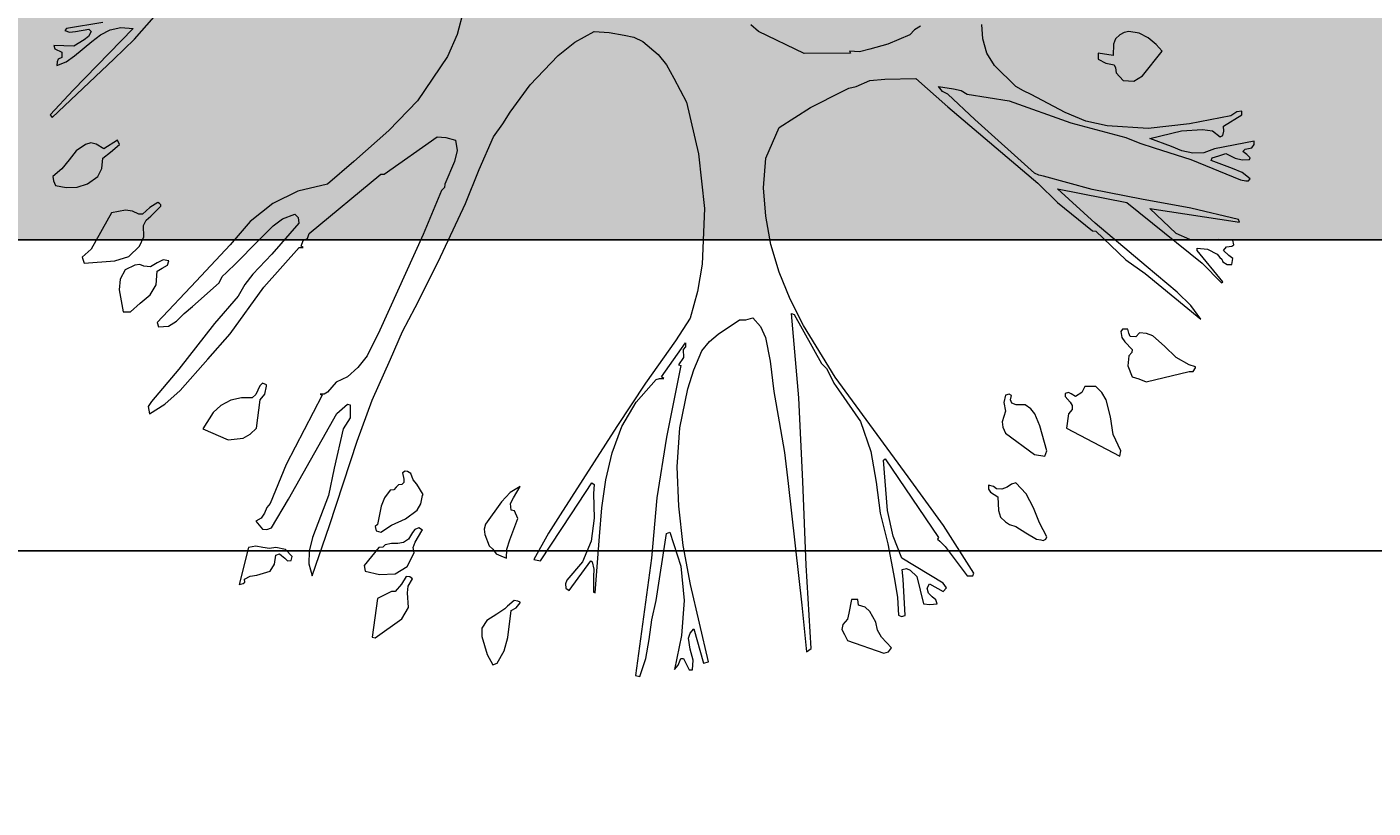
# Model space of a CAD drawing. Units: inches. Extents: x 84 to 1044, y -280 to 906.
# Tile 37 of 105: x 876 to 915, y -129 to -107. Entities that reach past the tile are written whole.
import ezdxf

# ---------------------------------------------------------------- set-up
doc = ezdxf.new("R2010")
doc.units = ezdxf.units.IN
for name, color, linetype, lineweight in [('A-ANNO-DIMS', 2, 'Continuous', 18), ('C-PROP', 7, 'Continuous', 25), ('L-PLNT', 114, 'Continuous', 15)]:
    doc.layers.add(name, color=color, linetype=linetype, lineweight=lineweight)
doc.layers.add('L-PLNT-PATT', color=9, linetype='Continuous', lineweight=9, true_color=0xafd9aa)
doc.styles.get("Standard").update_dxf_attribs({"font": 'arial.ttf'})
doc.dimstyles.get("Standard").update_dxf_attribs({"dimtxt": 0.18, "dimasz": 0.18, "dimexe": 0.18, "dimexo": 0.0625, "dimgap": 0.09, "dimtad": 0, "dimtih": 1, "dimtoh": 1, "dimdec": 4, "dimzin": 0, "dimdsep": 46, "dimtxsty": 'Standard', "dimcen": 0.09, "dimadec": 0, "dimazin": 0, "dimtfac": 1, "dimtdec": 4, "dimtofl": 0, "dimtmove": 0, "dimatfit": 3, "dimfxl": 1, "dimtolj": 1, "dimtzin": 0, "dimarcsym": 0})

# ---------------------------------------------------------------- blocks, each defined once
blk = doc.blocks.new('A$C37E508DF')
for p, q in [((0.9287, 0.7825), (0.936, 0.7542)), ((1.3151, 0.7487), (1.2919, 0.7752)), ((0.3186, 0.7491), (0.3199, 0.7662)), ((0.3919, 0.7641), (0.3988, 0.7598)), ((0.3988, 0.7598), (0.4043, 0.7538)), ((0.5823, 0.7577), (0.5913, 0.7658)), ((1.3309, 0.7624), (1.3164, 0.7615)), ((1.3164, 0.7615), (1.3871, 0.6891)), ((1.3434, 0.7598), (1.3309, 0.7624)), ((1.355, 0.7538), (1.3434, 0.7598)), ((1.352, 0.7684), (1.3948, 0.7615)), ((1.3687, 0.7607), (1.3657, 0.7577)), ((1.3841, 0.7577), (1.3687, 0.7607)), ((1.397, 0.759), (1.3914, 0.7572)), ((1.3948, 0.7615), (1.397, 0.759)), ((0.1153, 0.7427), (0.1244, 0.7504)), ((0.1244, 0.7504), (0.1351, 0.7559)), ((0.1351, 0.7559), (0.1471, 0.7577)), ((0.1471, 0.7577), (0.1527, 0.7568)), ((0.1527, 0.7568), (0.1578, 0.7538)), ((0.1578, 0.7538), (0.1629, 0.7491)), ((0.1629, 0.7491), (0.1651, 0.7431)), ((0.1651, 0.7431), (0.1655, 0.7298)), ((0.3139, 0.7324), (0.3186, 0.7491)), ((0.4043, 0.7538), (0.4301, 0.7431)), ((0.4301, 0.7431), (0.4515, 0.7371)), ((0.5287, 0.7319), (0.5823, 0.7577)), ((0.7182, 0.7461), (0.7002, 0.7307)), ((0.7285, 0.7512), (0.7182, 0.7461)), ((0.7401, 0.7534), (0.7285, 0.7512)), ((0.7577, 0.7568), (0.7401, 0.7534)), ((0.7752, 0.7577), (0.7577, 0.7568)), ((0.798, 0.7452), (0.7752, 0.7577)), ((0.8173, 0.7298), (0.798, 0.7452)), ((0.936, 0.7542), (0.9476, 0.7285)), ((1.3391, 0.7255), (1.3151, 0.7487)), ((1.3653, 0.7461), (1.355, 0.7538)), ((1.3854, 0.7294), (1.3653, 0.7461)), ((1.3657, 0.7577), (1.3691, 0.7521)), ((1.3691, 0.7521), (1.3743, 0.7482)), ((1.3743, 0.7482), (1.3863, 0.7405)), ((1.3914, 0.7572), (1.3841, 0.7577)), ((0.1081, 0.7349), (0.1153, 0.7427)), ((0.1312, 0.7058), (0.1081, 0.7349)), ((0.1655, 0.7298), (0.1831, 0.7324)), ((0.1831, 0.7324), (0.1831, 0.7255)), ((0.3049, 0.7178), (0.3139, 0.7324)), ((0.4515, 0.7371), (0.4635, 0.7341)), ((0.4635, 0.7341), (0.4755, 0.7349)), ((0.4755, 0.7349), (0.4742, 0.7324)), ((0.4742, 0.7324), (0.5287, 0.7319)), ((0.7002, 0.7307), (0.6903, 0.7186)), ((0.8344, 0.7122), (0.8173, 0.7298)), ((0.9476, 0.7285), (0.9828, 0.6762)), ((1.3953, 0.7221), (1.3854, 0.7294)), ((1.3863, 0.7405), (1.4099, 0.7414)), ((1.4086, 0.7375), (1.4004, 0.7337)), ((1.4004, 0.7337), (1.4004, 0.7272)), ((1.4004, 0.7272), (1.4047, 0.7255)), ((1.4099, 0.7414), (1.4086, 0.7375)), ((0.1629, 0.7152), (0.1621, 0.7092)), ((0.1646, 0.7186), (0.1629, 0.7152)), ((0.1741, 0.7208), (0.1646, 0.7186)), ((0.1831, 0.7255), (0.1741, 0.7208)), ((0.28, 0.6933), (0.3049, 0.7178)), ((0.6903, 0.7186), (0.6818, 0.7032)), ((0.8503, 0.6951), (0.8344, 0.7122)), ((1.4116, 0.6569), (1.3391, 0.7255)), ((1.4064, 0.7178), (1.3953, 0.7221)), ((1.4047, 0.7255), (1.406, 0.7221)), ((1.406, 0.7221), (1.4064, 0.7178)), ((0.1415, 0.6994), (0.1312, 0.7058)), ((0.1539, 0.7002), (0.1415, 0.6994)), ((0.1621, 0.7092), (0.1539, 0.7002)), ((0.3975, 0.7028), (0.3598, 0.6693)), ((0.4339, 0.7019), (0.3975, 0.7028)), ((0.4515, 0.7002), (0.4339, 0.7019)), ((0.4674, 0.6933), (0.4515, 0.7002)), ((0.6818, 0.7032), (0.6667, 0.6749)), ((0.2221, 0.6625), (0.262, 0.6839)), ((0.262, 0.6839), (0.271, 0.6882)), ((0.271, 0.6882), (0.28, 0.6933)), ((0.337, 0.6843), (0.2877, 0.6762)), ((0.328, 0.6543), (0.3598, 0.6843)), ((0.3443, 0.6886), (0.337, 0.6843)), ((0.3533, 0.6903), (0.3443, 0.6886)), ((0.3709, 0.6933), (0.3533, 0.6903)), ((0.3598, 0.6843), (0.3662, 0.6873)), ((0.3662, 0.6873), (0.3709, 0.6933)), ((0.476, 0.6912), (0.4674, 0.6933)), ((0.4832, 0.6878), (0.476, 0.6912)), ((0.521, 0.6685), (0.4832, 0.6878)), ((0.8739, 0.6629), (0.8503, 0.6951)), ((1.3871, 0.6891), (1.4141, 0.6599)), ((0.0146, 0.6599), (0.0146, 0.6642)), ((0.0146, 0.6642), (0.0206, 0.6633)), ((0.2877, 0.6762), (0.2152, 0.6505)), ((0.3598, 0.6693), (0.2543, 0.5797)), ((0.5578, 0.6449), (0.521, 0.6685)), ((0.6667, 0.6749), (0.6526, 0.614)), ((0.9828, 0.6762), (1.0162, 0.6415)), ((0.036, 0.6466), (0.0146, 0.6599)), ((0.0206, 0.6633), (0.0274, 0.6586)), ((0.0274, 0.6586), (0.0759, 0.6492)), ((0.0759, 0.6492), (0.1244, 0.644)), ((0.2152, 0.6505), (0.1509, 0.6333)), ((0.1728, 0.647), (0.1977, 0.6526)), ((0.1977, 0.6526), (0.2221, 0.6625)), ((0.2581, 0.5913), (0.328, 0.6543)), ((0.8824, 0.6492), (0.8739, 0.6629)), ((0.8932, 0.6342), (0.8824, 0.6492)), ((1.4141, 0.6599), (1.4116, 0.6569)), ((0.0356, 0.6406), (0.036, 0.6466)), ((0.0369, 0.6355), (0.0356, 0.6406)), ((0.0399, 0.6342), (0.0369, 0.6355)), ((0.0489, 0.641), (0.0399, 0.6342)), ((0.0609, 0.6428), (0.0489, 0.641)), ((0.0853, 0.641), (0.0609, 0.6428)), ((0.1226, 0.632), (0.0853, 0.641)), ((0.1244, 0.644), (0.1728, 0.647)), ((0.1509, 0.6333), (0.1342, 0.6265)), ((0.5737, 0.6089), (0.5578, 0.6449)), ((0.9103, 0.5956), (0.8932, 0.6342)), ((0.9493, 0.6333), (0.9382, 0.6303)), ((0.9596, 0.6342), (0.9493, 0.6333)), ((1.0218, 0.5904), (0.9596, 0.6342)), ((1.0162, 0.6415), (1.0574, 0.605)), ((0, 0.629), (0.0467, 0.62)), ((0, 0.6252), (0, 0.629)), ((0.003, 0.6213), (0, 0.6252)), ((0.0069, 0.6204), (0.003, 0.6213)), ((0.0107, 0.6196), (0.0069, 0.6204)), ((0.0086, 0.6132), (0.0133, 0.617)), ((0.0133, 0.617), (0.0107, 0.6196)), ((0.0467, 0.62), (0.0592, 0.6153)), ((0.072, 0.6149), (0.0849, 0.6175)), ((0.1175, 0.6213), (0.0746, 0.6076)), ((0.0849, 0.6175), (0.0973, 0.6226)), ((0.0973, 0.6226), (0.1226, 0.632)), ((0.1342, 0.6265), (0.1175, 0.6213)), ((0.9382, 0.6303), (0.936, 0.6179)), ((0.936, 0.6179), (0.939, 0.605)), ((1.3327, 0.6252), (1.3348, 0.6303)), ((1.343, 0.6162), (1.3327, 0.6252)), ((1.3348, 0.6303), (1.3511, 0.62)), ((1.3511, 0.62), (1.3601, 0.6256)), ((1.3601, 0.6256), (1.3661, 0.6269)), ((1.3661, 0.6269), (1.3725, 0.6252)), ((1.3725, 0.6252), (1.3837, 0.6175)), ((1.3837, 0.6175), (1.3918, 0.6072)), ((0.0047, 0.6093), (0.0086, 0.6132)), ((0.0056, 0.6076), (0.0047, 0.6093)), ((0.0141, 0.6072), (0.0056, 0.6076)), ((0.0223, 0.6089), (0.0141, 0.6072)), ((0.0746, 0.6076), (0.0163, 0.5836)), ((0.0334, 0.6145), (0.0223, 0.6089)), ((0.0257, 0.5969), (0.0506, 0.6063)), ((0.0416, 0.6119), (0.0334, 0.6145)), ((0.0493, 0.6093), (0.0416, 0.6119)), ((0.0506, 0.6063), (0.0493, 0.6093)), ((0.0592, 0.6153), (0.072, 0.6149)), ((0.5763, 0.5741), (0.5737, 0.6089)), ((0.6526, 0.614), (0.6457, 0.5497)), ((0.939, 0.605), (0.9506, 0.5784)), ((1.0574, 0.605), (1.0883, 0.5784)), ((1.352, 0.6089), (1.343, 0.6162)), ((1.3533, 0.5969), (1.352, 0.6089)), ((1.3918, 0.6072), (1.4004, 0.5964)), ((0.0047, 0.5849), (0.0141, 0.5921)), ((0.0141, 0.5921), (0.0257, 0.5969)), ((0.1904, 0.5724), (0.2474, 0.5879)), ((0.2474, 0.5879), (0.253, 0.5892)), ((0.253, 0.5892), (0.2581, 0.5913)), ((0.9262, 0.5557), (0.9103, 0.5956)), ((1.0256, 0.5904), (1.0218, 0.5904)), ((1.1097, 0.5205), (1.0256, 0.5904)), ((1.358, 0.5874), (1.3533, 0.5969)), ((1.37, 0.5789), (1.358, 0.5874)), ((1.4004, 0.5964), (1.4111, 0.5874)), ((1.4111, 0.5874), (1.4103, 0.5823)), ((0.0069, 0.5823), (0.0047, 0.5849)), ((0.0099, 0.5823), (0.0069, 0.5823)), ((0.0163, 0.5836), (0.0099, 0.5823)), ((0.1325, 0.5608), (0.1904, 0.5724)), ((0.2311, 0.5729), (0.1496, 0.557)), ((0.1869, 0.5325), (0.2311, 0.5729)), ((0.2543, 0.5797), (0.2311, 0.557)), ((0.5737, 0.5407), (0.5763, 0.5741)), ((0.9506, 0.5784), (0.951, 0.5746)), ((0.951, 0.5746), (0.9545, 0.5711)), ((0.9545, 0.5711), (0.9759, 0.5193)), ((1.0883, 0.5784), (1.123, 0.5703)), ((1.123, 0.5703), (1.1526, 0.5557)), ((1.3824, 0.575), (1.37, 0.5789)), ((1.3953, 0.5746), (1.3824, 0.575)), ((1.4077, 0.5771), (1.3953, 0.5746)), ((1.4103, 0.5823), (1.4077, 0.5771)), ((0.1496, 0.557), (0.0613, 0.4858)), ((0.0746, 0.5501), (0.1325, 0.5608)), ((0.2311, 0.557), (0.1899, 0.5235)), ((0.9583, 0.4871), (0.9262, 0.5557)), ((1.1526, 0.5557), (1.1792, 0.5347)), ((1.2842, 0.554), (1.2855, 0.5557)), ((1.2842, 0.5527), (1.2842, 0.554)), ((1.2855, 0.5557), (1.2876, 0.557)), ((1.2876, 0.557), (1.2971, 0.551)), ((0.1226, 0.5497), (0.0171, 0.5338)), ((0.0184, 0.5368), (0.0746, 0.5501)), ((0.0917, 0.5205), (0.1226, 0.5497)), ((0.5677, 0.5077), (0.5737, 0.5407)), ((0.6457, 0.5497), (0.6483, 0.4845)), ((1.1226, 0.5394), (1.1221, 0.5325)), ((1.1268, 0.5433), (1.1226, 0.5394)), ((1.141, 0.5377), (1.1268, 0.5433)), ((1.1521, 0.5296), (1.141, 0.5377)), ((1.2958, 0.5407), (1.2842, 0.5527)), ((1.3014, 0.536), (1.2958, 0.5407)), ((1.2971, 0.551), (1.3057, 0.5433)), ((1.3057, 0.5433), (1.3099, 0.5433)), ((1.3099, 0.5433), (1.3172, 0.5467)), ((1.3172, 0.5467), (1.3254, 0.548)), ((1.3254, 0.548), (1.3421, 0.5446)), ((1.3421, 0.5446), (1.3657, 0.5021)), ((0.0171, 0.5338), (0.0184, 0.5368)), ((0.1269, 0.482), (0.1869, 0.5325)), ((0.1861, 0.5231), (0.1509, 0.4897)), ((0.1899, 0.5235), (0.1861, 0.5231)), ((1.1221, 0.5325), (1.1539, 0.4961)), ((1.1706, 0.5111), (1.1521, 0.5296)), ((1.1792, 0.5347), (1.2027, 0.5072)), ((1.3044, 0.53), (1.3014, 0.536)), ((1.3039, 0.5167), (1.3044, 0.53)), ((0.024, 0.5072), (0.0253, 0.5128)), ((0.0262, 0.5055), (0.024, 0.5072)), ((0.0253, 0.5128), (0.042, 0.5133)), ((0.042, 0.5133), (0.0587, 0.5124)), ((0.0587, 0.5124), (0.0755, 0.5133)), ((0.0755, 0.5133), (0.0917, 0.5205)), ((0.5578, 0.4751), (0.5677, 0.5077)), ((0.9759, 0.5193), (1.0269, 0.4069)), ((1.1118, 0.5145), (1.1097, 0.5205)), ((1.117, 0.5124), (1.1118, 0.5145)), ((1.1191, 0.5055), (1.117, 0.5124)), ((1.1955, 0.4858), (1.1706, 0.5111)), ((1.2027, 0.5072), (1.2426, 0.4644)), ((1.3091, 0.5055), (1.3039, 0.5167)), ((0.0253, 0.491), (0.03, 0.4948)), ((0.0262, 0.4841), (0.0253, 0.491)), ((0.0326, 0.5047), (0.0262, 0.5055)), ((0.03, 0.4948), (0.036, 0.5004)), ((0.036, 0.5004), (0.0326, 0.5047)), ((0.0369, 0.4639), (0.0669, 0.5004)), ((0.0382, 0.4905), (0.0369, 0.4871)), ((0.0403, 0.4922), (0.0382, 0.4905)), ((0.0437, 0.4961), (0.0403, 0.4922)), ((0.0549, 0.5021), (0.0437, 0.4961)), ((0.0669, 0.5034), (0.0549, 0.5021)), ((0.0669, 0.5004), (0.0669, 0.5034)), ((1.117, 0.5042), (1.1191, 0.5055)), ((1.1217, 0.5042), (1.117, 0.5042)), ((1.1633, 0.4575), (1.1217, 0.5042)), ((1.1539, 0.4961), (1.1762, 0.4729)), ((1.3215, 0.4935), (1.3091, 0.5055)), ((1.3382, 0.4884), (1.3215, 0.4935)), ((1.3657, 0.5021), (1.3764, 0.4927)), ((1.3764, 0.4927), (1.3743, 0.4858)), ((0.0317, 0.4841), (0.0262, 0.4841)), ((0.0369, 0.4871), (0.0317, 0.4841)), ((0.0613, 0.4858), (0.0386, 0.4627)), ((0.0905, 0.4515), (0.1269, 0.482)), ((0.1509, 0.4897), (0.1282, 0.4734)), ((0.545, 0.4434), (0.5578, 0.4751)), ((0.6483, 0.4845), (0.6539, 0.4524)), ((0.9853, 0.4335), (0.9583, 0.4871)), ((1.207, 0.4747), (1.1955, 0.4858)), ((1.2122, 0.47), (1.207, 0.4747)), ((1.2748, 0.4884), (1.2812, 0.4897)), ((1.2761, 0.4832), (1.2748, 0.4884)), ((1.2825, 0.4798), (1.2761, 0.4832)), ((1.2812, 0.4897), (1.2885, 0.4862)), ((1.2885, 0.4764), (1.2825, 0.4798)), ((1.2885, 0.4862), (1.2962, 0.4815)), ((1.2894, 0.4601), (1.2885, 0.4764)), ((1.2962, 0.4815), (1.3039, 0.482)), ((1.3039, 0.482), (1.3087, 0.4841)), ((1.3087, 0.4841), (1.3147, 0.4832)), ((1.3147, 0.4832), (1.3258, 0.4777)), ((1.3258, 0.4777), (1.3318, 0.4669)), ((1.3743, 0.4858), (1.3382, 0.4884)), ((0.0386, 0.4627), (0.0369, 0.4639)), ((0.1282, 0.4734), (0.0626, 0.4198)), ((1.1762, 0.4729), (1.1856, 0.4605)), ((1.1856, 0.4605), (1.1933, 0.4468)), ((1.2156, 0.4627), (1.2122, 0.47)), ((1.2469, 0.4348), (1.2156, 0.4627)), ((1.2426, 0.4644), (1.2885, 0.4159)), ((1.2967, 0.4485), (1.2894, 0.4601)), ((1.3318, 0.4669), (1.3331, 0.4545)), ((0.0746, 0.4361), (0.0905, 0.4515)), ((0.5295, 0.4125), (0.545, 0.4434)), ((0.6539, 0.4524), (0.6625, 0.4211)), ((1.2027, 0.4026), (1.1633, 0.4575)), ((1.1933, 0.4468), (1.2212, 0.4146)), ((1.3082, 0.4386), (1.2967, 0.4485)), ((1.3331, 0.4545), (1.3284, 0.4284)), ((0.0626, 0.4198), (0.0746, 0.4361)), ((1.0003, 0.4052), (0.9853, 0.4335)), ((1.2568, 0.4266), (1.2469, 0.4348)), ((1.3198, 0.4284), (1.3082, 0.4386)), ((1.3284, 0.4284), (1.3198, 0.4284)), ((0.4922, 0.3516), (0.5295, 0.4125)), ((0.5403, 0.4254), (0.5081, 0.3679)), ((0.5347, 0.3276), (0.5433, 0.4266)), ((0.5433, 0.4266), (0.5403, 0.4254)), ((0.5797, 0.4112), (0.5741, 0.3983)), ((0.5887, 0.4215), (0.5797, 0.4112)), ((0.5969, 0.4189), (0.5887, 0.4215)), ((0.6046, 0.4189), (0.5969, 0.4189)), ((0.6295, 0.4022), (0.6046, 0.4189)), ((0.6625, 0.4211), (0.6796, 0.3945)), ((1.2212, 0.4146), (1.2628, 0.361)), ((1.2658, 0.4176), (1.2568, 0.4266)), ((1.2752, 0.4116), (1.2658, 0.4176)), ((1.2868, 0.4108), (1.2752, 0.4116)), ((1.2885, 0.4159), (1.2868, 0.4108)), ((0.1055, 0.388), (0.1192, 0.4001)), ((0.1192, 0.4001), (0.1265, 0.4031)), ((0.1265, 0.4031), (0.1346, 0.4039)), ((0.1346, 0.4039), (0.1389, 0.3992)), ((0.1389, 0.3992), (0.1458, 0.3996)), ((0.1458, 0.3996), (0.1471, 0.4035)), ((0.1471, 0.4035), (0.1484, 0.4082)), ((0.1484, 0.4082), (0.1548, 0.4082)), ((0.1556, 0.3983), (0.1518, 0.3932)), ((0.1548, 0.4082), (0.1565, 0.4052)), ((0.1565, 0.4052), (0.1556, 0.3983)), ((0.5741, 0.3983), (0.5686, 0.3705)), ((0.6397, 0.3936), (0.6295, 0.4022)), ((1.0145, 0.373), (1.0003, 0.4052)), ((1.0269, 0.4069), (1.0419, 0.3769)), ((1.2289, 0.373), (1.2027, 0.4026)), ((0.0917, 0.3748), (0.1055, 0.388)), ((0.1518, 0.3932), (0.1432, 0.3842)), ((0.1432, 0.3842), (0.1436, 0.3808)), ((0.1436, 0.3808), (0.1471, 0.3769)), ((0.6487, 0.3825), (0.6397, 0.3936)), ((0.6582, 0.3602), (0.6487, 0.3825)), ((0.6959, 0.352), (0.668, 0.3919)), ((0.668, 0.3919), (0.668, 0.3872)), ((0.668, 0.3872), (0.6706, 0.3842)), ((0.6706, 0.3842), (0.6702, 0.3748)), ((0.6796, 0.3945), (0.7148, 0.3447)), ((0.069, 0.364), (0.0763, 0.3662)), ((0.069, 0.3627), (0.069, 0.364)), ((0.0763, 0.3662), (0.0917, 0.3748)), ((0.1484, 0.3649), (0.1432, 0.352)), ((0.1471, 0.3769), (0.1484, 0.3649)), ((0.5081, 0.3679), (0.5025, 0.3619)), ((0.5686, 0.3705), (0.5643, 0.3349)), ((0.6702, 0.3748), (0.6762, 0.3662)), ((0.6762, 0.3662), (0.6732, 0.3653)), ((0.6732, 0.3653), (0.6903, 0.2813)), ((1.0359, 0.3246), (1.0145, 0.373)), ((1.0419, 0.3769), (1.0527, 0.3632)), ((1.2615, 0.3362), (1.2289, 0.373)), ((0.0716, 0.3585), (0.069, 0.3627)), ((0.0763, 0.3585), (0.0716, 0.3585)), ((0.1269, 0.3464), (0.0763, 0.3585)), ((0.1355, 0.3499), (0.1269, 0.3464)), ((0.1432, 0.352), (0.1355, 0.3499)), ((0.4065, 0.2345), (0.4922, 0.3516)), ((0.4982, 0.3537), (0.4939, 0.3447)), ((0.5025, 0.3619), (0.4982, 0.3537)), ((0.665, 0.3379), (0.6582, 0.3602)), ((0.6933, 0.3503), (0.6959, 0.352)), ((0.6985, 0.3503), (0.6933, 0.3503)), ((0.7023, 0.349), (0.6985, 0.3503)), ((0.7259, 0.3224), (0.7023, 0.349)), ((1.0527, 0.3632), (1.0647, 0.352)), ((1.0647, 0.352), (1.078, 0.346)), ((1.2628, 0.361), (1.2949, 0.3233)), ((0.1737, 0.325), (0.1788, 0.3336)), ((0.1788, 0.3336), (0.1861, 0.3409)), ((0.1861, 0.3409), (0.199, 0.3409)), ((0.199, 0.3409), (0.2024, 0.3336)), ((0.2024, 0.3336), (0.2097, 0.3289)), ((0.2097, 0.3289), (0.2148, 0.3323)), ((0.2148, 0.3323), (0.2182, 0.3336)), ((0.2182, 0.3336), (0.2221, 0.3327)), ((0.2221, 0.3327), (0.2221, 0.3289)), ((0.4884, 0.337), (0.4622, 0.2997)), ((0.4939, 0.3447), (0.4884, 0.337)), ((0.5643, 0.3349), (0.5578, 0.2993)), ((0.6745, 0.2924), (0.665, 0.3379)), ((0.7148, 0.3447), (0.7487, 0.2937)), ((1.078, 0.346), (1.0883, 0.334)), ((1.0883, 0.334), (1.0921, 0.3319)), ((1.1599, 0.3426), (1.1646, 0.3447)), ((1.1599, 0.3413), (1.1599, 0.3426)), ((1.162, 0.3319), (1.1599, 0.3413)), ((1.1646, 0.3447), (1.168, 0.3417)), ((1.168, 0.3417), (1.1702, 0.3366)), ((1.1702, 0.3366), (1.1727, 0.3314)), ((1.2795, 0.3199), (1.2615, 0.3362)), ((0.1689, 0.3053), (0.1737, 0.325)), ((0.2161, 0.3224), (0.214, 0.3186)), ((0.214, 0.3186), (0.214, 0.3139)), ((0.2221, 0.3289), (0.2161, 0.3224)), ((0.2624, 0.3147), (0.2689, 0.3194)), ((0.2689, 0.3194), (0.2796, 0.3194)), ((0.2796, 0.3194), (0.2847, 0.3211)), ((0.2847, 0.3211), (0.2864, 0.325)), ((0.2851, 0.3302), (0.2877, 0.3319)), ((0.2864, 0.325), (0.2851, 0.3302)), ((0.2877, 0.3319), (0.292, 0.3306)), ((0.292, 0.3306), (0.2941, 0.322)), ((0.2941, 0.322), (0.292, 0.3117)), ((0.53, 0.229), (0.5347, 0.3276)), ((0.7427, 0.2937), (0.7259, 0.3224)), ((1.0535, 0.2766), (1.0359, 0.3246)), ((1.0647, 0.3199), (1.0617, 0.3194)), ((1.0617, 0.3194), (1.0617, 0.304)), ((1.0711, 0.3147), (1.0647, 0.3199)), ((1.0921, 0.3319), (1.0968, 0.3319)), ((1.0968, 0.3319), (1.0947, 0.3306)), ((1.0947, 0.3306), (1.1367, 0.2491)), ((1.1676, 0.325), (1.162, 0.3319)), ((1.1719, 0.292), (1.1676, 0.325)), ((1.1727, 0.3314), (1.177, 0.3276)), ((1.177, 0.3276), (1.1895, 0.3276)), ((1.1895, 0.3276), (1.2019, 0.3246)), ((1.2019, 0.3246), (1.2135, 0.3186)), ((1.2135, 0.3186), (1.2225, 0.3104)), ((1.2975, 0.3087), (1.2795, 0.3199)), ((1.2949, 0.3233), (1.2988, 0.3173)), ((1.2988, 0.3173), (1.2975, 0.3087)), ((0.1655, 0.2843), (0.1689, 0.3053)), ((0.214, 0.3139), (0.2182, 0.3087)), ((0.2182, 0.3087), (0.2204, 0.292)), ((0.2517, 0.2946), (0.2577, 0.3087)), ((0.2577, 0.3087), (0.2624, 0.3147)), ((0.292, 0.3117), (0.2959, 0.2993)), ((1.0617, 0.304), (1.0698, 0.2911)), ((1.0775, 0.3092), (1.0711, 0.3147)), ((1.1341, 0.2084), (1.0775, 0.3092)), ((1.2225, 0.3104), (1.2349, 0.2911)), ((0.2204, 0.292), (0.1578, 0.259)), ((0.2436, 0.265), (0.2517, 0.2946)), ((0.292, 0.286), (0.2581, 0.2607)), ((0.2954, 0.2928), (0.292, 0.286)), ((0.2959, 0.2993), (0.2954, 0.2928)), ((0.4622, 0.2997), (0.4502, 0.2645)), ((0.5578, 0.2993), (0.5518, 0.2633)), ((0.6775, 0.2465), (0.6745, 0.2924)), ((0.7542, 0.2628), (0.7427, 0.2937)), ((0.7487, 0.2937), (0.8151, 0.1899)), ((1.0698, 0.2911), (1.0805, 0.2448)), ((1.1792, 0.2847), (1.1719, 0.292)), ((1.1873, 0.28), (1.1792, 0.2847)), ((1.2349, 0.2911), (1.2049, 0.2783)), ((0.1565, 0.265), (0.1655, 0.2843)), ((0.6903, 0.2813), (0.7015, 0.2101)), ((1.0861, 0.1775), (1.0535, 0.2766)), ((1.2049, 0.2783), (1.1873, 0.28)), ((0.1578, 0.259), (0.1565, 0.265)), ((0.2461, 0.259), (0.2436, 0.265)), ((0.2581, 0.2607), (0.2461, 0.259)), ((0.4335, 0.2556), (0.3709, 0.1634)), ((0.4305, 0.1951), (0.4352, 0.2543)), ((0.4352, 0.2543), (0.4335, 0.2556)), ((0.4502, 0.2645), (0.4438, 0.2285)), ((0.5518, 0.2633), (0.5475, 0.2268)), ((0.7615, 0.2311), (0.7542, 0.2628)), ((0.6758, 0.2002), (0.6775, 0.2465)), ((0.9879, 0.2311), (0.9905, 0.2384)), ((0.9905, 0.2384), (0.9943, 0.241)), ((0.9943, 0.241), (0.9973, 0.2414)), ((0.9973, 0.2414), (1.0003, 0.2393)), ((1.0003, 0.2393), (0.9986, 0.232)), ((1.0805, 0.2448), (1.087, 0.2127)), ((1.1367, 0.2491), (1.1556, 0.2032)), ((0.268, 0.2148), (0.28, 0.2277)), ((0.28, 0.2277), (0.2851, 0.226)), ((0.2851, 0.226), (0.2903, 0.2225)), ((0.2903, 0.2225), (0.2963, 0.22)), ((0.3027, 0.2204), (0.3061, 0.2234)), ((0.3061, 0.2234), (0.3122, 0.2247)), ((0.3122, 0.2247), (0.3122, 0.22)), ((0.3649, 0.1775), (0.4065, 0.2345)), ((0.4438, 0.2285), (0.4391, 0.1921)), ((0.5261, 0.1308), (0.53, 0.229)), ((0.5475, 0.2268), (0.5313, 0.084)), ((0.7662, 0.1981), (0.7615, 0.2311)), ((0.7778, 0.2277), (0.7752, 0.2255)), ((0.7752, 0.2255), (0.7761, 0.2152)), ((0.8018, 0.1912), (0.7778, 0.2277)), ((0.8619, 0.2234), (0.8739, 0.2161)), ((0.87, 0.2101), (0.8619, 0.2234)), ((0.9759, 0.214), (0.9836, 0.226)), ((0.9836, 0.226), (0.9879, 0.2311)), ((0.9986, 0.232), (0.9986, 0.2281)), ((0.9986, 0.2281), (1.0012, 0.2255)), ((1.0012, 0.2255), (1.0051, 0.2251)), ((1.0051, 0.2251), (1.0076, 0.2225)), ((1.0076, 0.2225), (1.0106, 0.2195)), ((0.2594, 0.1981), (0.268, 0.2148)), ((0.2963, 0.22), (0.3027, 0.2204)), ((0.301, 0.211), (0.3002, 0.1951)), ((0.3096, 0.2165), (0.301, 0.211)), ((0.3122, 0.22), (0.3096, 0.2165)), ((0.7015, 0.2101), (0.7079, 0.1389)), ((0.7761, 0.2152), (0.7752, 0.1861)), ((0.8734, 0.2032), (0.87, 0.2101)), ((0.8739, 0.2161), (0.8841, 0.2054)), ((0.9768, 0.2127), (0.9759, 0.214)), ((0.9789, 0.2028), (0.9768, 0.2127)), ((1.0106, 0.2195), (1.0149, 0.2191)), ((1.0149, 0.2191), (1.0214, 0.2101)), ((1.0214, 0.2101), (1.0252, 0.2002)), ((1.087, 0.2127), (1.0998, 0.1797)), ((1.1543, 0.1749), (1.1341, 0.2084)), ((0.2521, 0.1805), (0.2594, 0.1981)), ((0.3002, 0.1951), (0.298, 0.1874)), ((0.4241, 0.1651), (0.4305, 0.1951)), ((0.4391, 0.1921), (0.4301, 0.1561)), ((0.6706, 0.1539), (0.6758, 0.2002)), ((0.7688, 0.1646), (0.7662, 0.1981)), ((0.8383, 0.1359), (0.8018, 0.1912)), ((0.8151, 0.1899), (0.8288, 0.1685)), ((0.8649, 0.1857), (0.8687, 0.1947)), ((0.8687, 0.1947), (0.8726, 0.1955)), ((0.8726, 0.1955), (0.8734, 0.2032)), ((0.8841, 0.2054), (0.9026, 0.1792)), ((0.9832, 0.1955), (0.9789, 0.2028)), ((0.9969, 0.1852), (0.9832, 0.1955)), ((1.0252, 0.2002), (1.0295, 0.1788)), ((1.1556, 0.2032), (1.1594, 0.1985)), ((1.1594, 0.1985), (1.1624, 0.1921)), ((1.1624, 0.1921), (1.1663, 0.1861)), ((0.2436, 0.1642), (0.2521, 0.1805)), ((0.28, 0.1762), (0.2684, 0.1689)), ((0.2873, 0.1788), (0.28, 0.1762)), ((0.292, 0.1818), (0.2873, 0.1788)), ((0.298, 0.1874), (0.292, 0.1818)), ((0.3293, 0.1213), (0.3649, 0.1775)), ((0.7752, 0.1861), (0.7787, 0.1591)), ((0.8743, 0.1608), (0.8649, 0.1857)), ((0.9026, 0.1792), (0.9043, 0.1732)), ((0.9768, 0.1719), (0.9811, 0.1749)), ((0.9811, 0.1749), (0.9858, 0.1728)), ((1.0132, 0.1779), (0.9969, 0.1852)), ((1.0256, 0.1698), (1.0132, 0.1779)), ((1.0295, 0.1788), (1.0325, 0.1762)), ((1.0325, 0.1762), (1.0312, 0.1711)), ((1.1063, 0.1183), (1.0861, 0.1775)), ((1.0998, 0.1797), (1.1058, 0.1634)), ((1.1594, 0.1728), (1.1543, 0.1749)), ((1.1727, 0.1827), (1.1646, 0.1732)), ((1.1663, 0.1861), (1.1727, 0.1827)), ((0.2448, 0.1616), (0.2436, 0.1642)), ((0.2478, 0.1599), (0.2448, 0.1616)), ((0.2508, 0.1608), (0.2478, 0.1599)), ((0.2556, 0.1616), (0.2508, 0.1608)), ((0.2684, 0.1689), (0.2556, 0.1616)), ((0.3692, 0.1591), (0.3628, 0.1526)), ((0.3718, 0.1616), (0.3692, 0.1591)), ((0.3709, 0.1634), (0.3718, 0.1616)), ((0.4138, 0.1389), (0.4241, 0.1651)), ((0.6865, 0.1698), (0.6732, 0.1295)), ((0.6903, 0.1681), (0.6865, 0.1698)), ((0.7023, 0.0892), (0.6903, 0.1681)), ((0.774, 0.0982), (0.7688, 0.1646)), ((0.7787, 0.1591), (0.789, 0.1346)), ((0.8288, 0.1685), (0.846, 0.1376)), ((0.8777, 0.1496), (0.8743, 0.1608)), ((0.9035, 0.1668), (0.8983, 0.1535)), ((0.9043, 0.1732), (0.9035, 0.1668)), ((0.9776, 0.1711), (0.9768, 0.1719)), ((0.9853, 0.1578), (0.9776, 0.1711)), ((0.9858, 0.1728), (0.9884, 0.1694)), ((0.9884, 0.1694), (0.9931, 0.1616)), ((0.9931, 0.1616), (0.9991, 0.1574)), ((1.0312, 0.1711), (1.0256, 0.1698)), ((1.1058, 0.1634), (1.1097, 0.1475)), ((1.1646, 0.1732), (1.1594, 0.1728)), ((0.3628, 0.1526), (0.337, 0.1183)), ((0.4301, 0.1561), (0.4224, 0.1145)), ((0.662, 0.108), (0.6706, 0.1539)), ((0.8781, 0.1389), (0.8777, 0.1496)), ((0.8902, 0.1441), (0.8846, 0.1419)), ((0.894, 0.1496), (0.8902, 0.1441)), ((0.8983, 0.1535), (0.894, 0.1496)), ((0.9879, 0.1518), (0.9853, 0.1578)), ((0.9866, 0.1453), (0.9879, 0.1518)), ((0.9948, 0.1291), (0.9866, 0.1453)), ((0.9991, 0.1574), (1.0059, 0.1565)), ((1.0059, 0.1565), (1.0132, 0.1565)), ((1.0132, 0.1565), (1.0205, 0.1548)), ((1.0205, 0.1548), (1.0235, 0.1522)), ((1.0235, 0.1522), (1.0282, 0.1518)), ((1.0282, 0.1518), (1.0454, 0.1303)), ((1.1097, 0.1475), (1.1101, 0.1325)), ((1.1298, 0.1411), (1.1376, 0.1492)), ((1.1376, 0.1492), (1.1491, 0.1518)), ((1.1423, 0.1423), (1.1384, 0.1389)), ((1.1449, 0.1441), (1.1423, 0.1423)), ((1.1491, 0.1428), (1.1449, 0.1441)), ((1.1491, 0.1518), (1.1564, 0.1505)), ((1.1504, 0.132), (1.1491, 0.1428)), ((1.1564, 0.1505), (1.1642, 0.1518)), ((1.1642, 0.1518), (1.1727, 0.1531)), ((1.1727, 0.1531), (1.1813, 0.1518)), ((1.1813, 0.1518), (1.192, 0.108)), ((0.3653, 0.1098), (0.4138, 0.1389)), ((0.4082, 0.1269), (0.4039, 0.1248)), ((0.4134, 0.1256), (0.4082, 0.1269)), ((0.5205, 0.033), (0.5261, 0.1308)), ((0.6732, 0.1295), (0.6693, 0.0892)), ((0.7079, 0.1389), (0.7268, 0.0013)), ((0.7774, 0.1346), (0.7757, 0.1261)), ((0.7791, 0.1359), (0.7774, 0.1346)), ((0.8044, 0.1012), (0.7791, 0.1359)), ((0.789, 0.1346), (0.8074, 0.1132)), ((0.846, 0.1376), (0.8383, 0.1359)), ((0.8846, 0.1419), (0.8781, 0.1389)), ((1.0089, 0.1205), (0.9948, 0.1291)), ((1.0454, 0.1303), (1.0441, 0.1239)), ((1.1101, 0.1325), (1.1063, 0.1183)), ((1.1311, 0.1364), (1.1298, 0.1411)), ((1.1354, 0.1359), (1.1311, 0.1364)), ((1.1384, 0.1389), (1.1354, 0.1359)), ((1.1556, 0.1239), (1.1504, 0.132)), ((0.3306, 0.1183), (0.3293, 0.1213)), ((0.337, 0.1183), (0.3306, 0.1183)), ((0.3962, 0.1175), (0.3885, 0.0853)), ((0.4039, 0.1248), (0.3962, 0.1175)), ((0.4099, 0.0716), (0.4121, 0.1145)), ((0.4121, 0.1145), (0.4134, 0.1256)), ((0.4224, 0.1145), (0.4189, 0.093)), ((0.7757, 0.1261), (0.7761, 0.117)), ((0.7761, 0.117), (0.7761, 0.099)), ((0.8074, 0.1132), (0.8087, 0.1089)), ((0.9884, 0.1149), (0.9918, 0.117)), ((0.9935, 0.1063), (0.9884, 0.1149)), ((0.9918, 0.117), (0.9961, 0.1175)), ((0.9961, 0.1175), (1.0016, 0.1085)), ((1.0274, 0.12), (1.0089, 0.1205)), ((1.0441, 0.1239), (1.0274, 0.12)), ((1.1714, 0.1192), (1.1556, 0.1239)), ((1.1792, 0.1179), (1.1714, 0.1192)), ((1.186, 0.1145), (1.1792, 0.1179)), ((1.1856, 0.111), (1.186, 0.1145)), ((1.1873, 0.1093), (1.1856, 0.111)), ((0.3615, 0.1042), (0.3653, 0.1098)), ((0.3653, 0.0999), (0.3615, 0.1042)), ((0.3812, 0.1089), (0.3653, 0.0999)), ((0.3782, 0.0935), (0.3825, 0.0978)), ((0.3842, 0.1037), (0.3812, 0.1089)), ((0.3825, 0.0978), (0.3842, 0.1037)), ((0.641, 0.0172), (0.662, 0.108)), ((0.7761, 0.099), (0.774, 0.0982)), ((0.8083, 0.1037), (0.8044, 0.1012)), ((0.8087, 0.1089), (0.8083, 0.1037)), ((0.9931, 0.081), (0.9943, 0.0982)), ((0.9943, 0.0982), (0.9935, 0.1063)), ((1.0016, 0.1085), (1.0089, 0.0999)), ((1.0089, 0.0999), (1.0132, 0.0999)), ((1.0132, 0.0999), (1.0295, 0.0917)), ((1.192, 0.108), (1.1873, 0.1093)), ((0.3722, 0.0853), (0.3739, 0.09)), ((0.3808, 0.0845), (0.3722, 0.0853)), ((0.3739, 0.09), (0.3782, 0.0935)), ((0.3885, 0.0853), (0.3808, 0.0845)), ((0.4189, 0.093), (0.4176, 0.072)), ((0.4515, 0.0763), (0.4571, 0.0815)), ((0.4571, 0.0815), (0.4648, 0.084)), ((0.4648, 0.084), (0.4657, 0.0905)), ((0.4657, 0.0905), (0.473, 0.0905)), ((0.473, 0.0905), (0.476, 0.0746)), ((0.5313, 0.084), (0.5257, 0.0291)), ((0.6693, 0.0892), (0.6728, 0.0484)), ((0.7075, 0.0665), (0.7023, 0.0892)), ((0.8619, 0.0875), (0.8649, 0.0887)), ((0.8619, 0.0866), (0.8619, 0.0875)), ((0.8666, 0.0806), (0.8619, 0.0866)), ((0.8649, 0.0887), (0.8691, 0.0892)), ((0.8726, 0.0776), (0.8666, 0.0806)), ((0.8691, 0.0892), (0.8769, 0.0827)), ((0.8769, 0.0827), (0.8799, 0.0797)), ((0.8799, 0.0797), (0.8893, 0.0733)), ((1.0012, 0.0677), (0.9931, 0.081)), ((1.0295, 0.0917), (1.0359, 0.0463)), ((0.4142, 0.0707), (0.4099, 0.0716)), ((0.4176, 0.072), (0.4142, 0.0707)), ((0.4425, 0.0544), (0.4442, 0.0639)), ((0.4442, 0.0639), (0.4515, 0.0763)), ((0.476, 0.0746), (0.4777, 0.0673)), ((0.4777, 0.0673), (0.4832, 0.0613)), ((0.7105, 0.0437), (0.7075, 0.0665)), ((0.8764, 0.0459), (0.8726, 0.0776)), ((0.8893, 0.0733), (0.9013, 0.066)), ((0.9013, 0.066), (0.9069, 0.057)), ((1.0325, 0.0454), (1.0012, 0.0677)), ((0.4378, 0.0463), (0.4425, 0.0544)), ((0.4811, 0.0493), (0.4777, 0.0424)), ((0.4845, 0.0553), (0.4811, 0.0493)), ((0.4832, 0.0613), (0.4845, 0.0553)), ((0.6582, 0.0562), (0.6466, 0.0159)), ((0.6625, 0.051), (0.6582, 0.0562)), ((0.6642, 0.045), (0.6625, 0.051)), ((0.6728, 0.0484), (0.6809, 0.0082)), ((0.9069, 0.057), (0.9069, 0.0471)), ((0.4258, 0.0339), (0.4378, 0.0463)), ((0.4296, 0.0291), (0.4258, 0.0339)), ((0.4777, 0.0424), (0.4348, 0.0274)), ((0.5257, 0.0291), (0.5205, 0.033)), ((0.659, 0.0193), (0.6625, 0.0321)), ((0.6625, 0.0321), (0.6642, 0.045)), ((0.7144, 0.0214), (0.7105, 0.0437)), ((0.8807, 0.0304), (0.8764, 0.0459)), ((0.9069, 0.0471), (0.9009, 0.0261)), ((1.0359, 0.0463), (1.0325, 0.0454)), ((0.4348, 0.0274), (0.4296, 0.0291)), ((0.6466, 0.0159), (0.641, 0.0172)), ((0.6595, 0.0077), (0.659, 0.0193)), ((0.6702, 0.0214), (0.6637, 0.0077)), ((0.6732, 0.0214), (0.6702, 0.0214)), ((0.6766, 0.0133), (0.6732, 0.0214)), ((0.7216, 0), (0.7144, 0.0214)), ((0.8889, 0.0159), (0.8807, 0.0304)), ((0.894, 0.0137), (0.8889, 0.0159)), ((0.9009, 0.0261), (0.894, 0.0137)), ((0.6637, 0.0077), (0.6595, 0.0077)), ((0.6809, 0.0082), (0.6766, 0.0133)), ((0.7268, 0.0013), (0.7216, 0))]:
    blk.add_line(p, q)
blk = doc.blocks.new('*D60')
at = {"layer": 'A-ANNO-DIMS', "color": 0, "lineweight": -2, "transparency": 16777216}
for p, q in [((134.179, -121.942), (134.179, -180.64)), ((992.074, -121.942), (992.074, -180.64)), ((134.359, -180.46), (562.733, -180.46)), ((991.894, -180.46), (563.521, -180.46))]:
    blk.add_line(p, q, dxfattribs=at)
at = {"layer": 'A-ANNO-DIMS', "color": 0, "transparency": 16777216}
for points in [[(134.359, -180.43), (134.359, -180.49), (134.179, -180.46)], [(991.894, -180.43), (991.894, -180.49), (992.074, -180.46)]]:
    blk.add_solid(points, dxfattribs=at)
at = {"layer": 'Defpoints', "color": 0, "transparency": 16777216}
for p in [(134.179, -121.88), (992.074, -121.88), (992.074, -180.46)]:
    blk.add_point(p, dxfattribs=at)
at = {"layer": 'A-ANNO-DIMS', "color": 0, "transparency": 16777216, "insert": (563.127, -180.46), "char_height": 0.18, "attachment_point": 5}
blk.add_mtext('\\A1;857.9', dxfattribs=at)

msp = doc.modelspace()

# ---------------------------------------------------------------- hatches: boundary and pattern name
at = {"layer": 'L-PLNT-PATT', "transparency": 33554597}
h = msp.add_hatch(color=256, dxfattribs=at)
h.dxf.hatch_style = 1
h.paths.add_polyline_path([(791.074, 31.12), (791.074, 91.12), (743.074, 91.12), (674.074, 91.12), (674.074, 31.12), (650.074, 31.12), (650.074, -112.88), (983.074, -112.88), (983.074, -64.88), (791.074, -64.88)])

# ---------------------------------------------------------------- linework, layer by layer
at = {"layer": 'C-PROP'}
for points in [[(143.179, -121.88), (134.179, -121.88), (134.179, 856.12), (992.074, 856.12), (992.074, -121.88), (624.574, -121.88)], [(143.179, -112.88), (143.179, 847.12), (983.074, 847.12), (983.074, -112.88), (624.574, -112.88)]]:
    msp.add_lwpolyline(points, dxfattribs=at)

# ---------------------------------------------------------------- block references
at = {"layer": 'L-PLNT', "xscale": -24.64361536662419, "yscale": 24.64361536662419, "zscale": 24.64361536662419}
msp.add_blockref('A$C37E508DF', (911.469, -125.52), dxfattribs=at)

# ---------------------------------------------------------------- dimensions: what is measured, and where the dimension line sits
at = {"layer": 'A-ANNO-DIMS'}
dim = msp.add_linear_dim(base=(992.074, -180.46), p1=(134.179, -121.88), p2=(992.074, -121.88), dimstyle='Standard', override={"dimdec": 1, "dimlfac": 1, "dimrnd": 0, "dimzin": 0, "dimdsep": 46, "dimlunit": 2}, dxfattribs=at)
dim.commit()
dim.dimension.update_dxf_attribs({"geometry": '*D60', "text_midpoint": (563.127, -180.46)})

doc.saveas('drawing.dxf')
